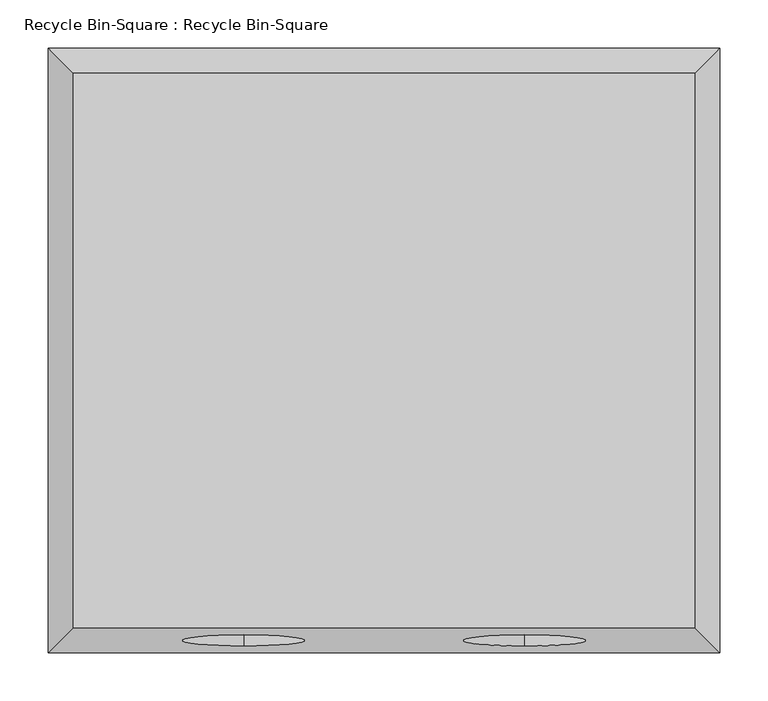
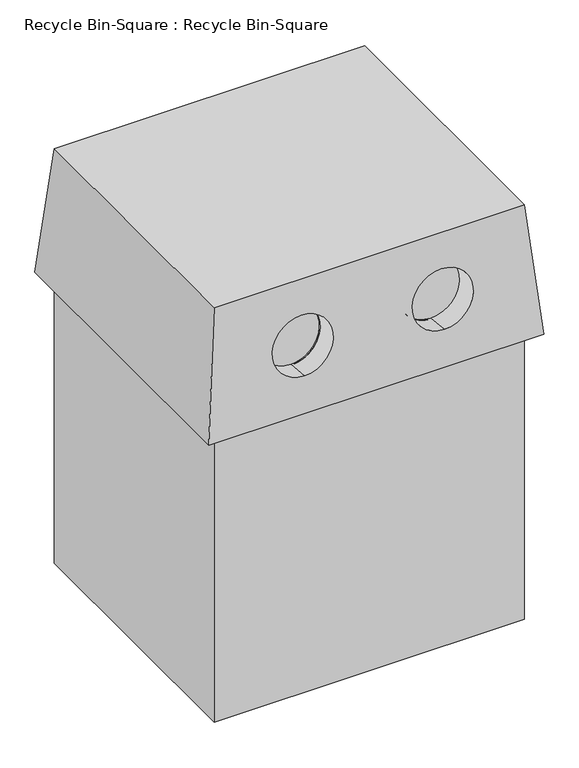
"""IFC4 building model written with IfcOpenShell, lengths in millimetres: proxy geometry, Recycle Bin-Square : Recycle Bin-Square."""

from ifc_helpers import new_model, si_unit, point, frame, frame_2d, origin, origin_with_axes, place, context, project, spatial, polyline, circle_curve, ellipse_curve, trimmed, segment, composite_curve, outline, extrude, source, transform, mapped, element, save
from ifc_brep_helpers import plane_surface, revolved_surface, advanced_brep


def recycle_bin_square_recycle_bin_square_c944da42(model_context):
    return source(origin(), model_context, "Body", "SolidModel", [
        extrude(outline(composite_curve([segment(trimmed(circle_curve(frame_2d((0.0, -63.5)), 63.5), [point((0.0, -127.0))], [point((0.0, 0.0))], False, "CARTESIAN"), True, "CONTINUOUS"), segment(trimmed(circle_curve(frame_2d((0.0, -63.5)), 63.5), [point((0.0, 0.0))], [point((6.35, -0.3182978))], False, "CARTESIAN"), True, "CONTINUOUS"), segment(trimmed(circle_curve(frame_2d((12.7, -63.5)), 63.5), [point((6.35, -0.3182978))], [point((6.35, -126.6817023))], True, "CARTESIAN"), True, "CONTINUOUS"), segment(trimmed(circle_curve(frame_2d((0.0, -63.5)), 63.5), [point((6.35, -126.6817023))], [point((0.0, -127.0))], False, "CARTESIAN"), True, "CONTINUOUS")], self_intersect=False)), frame((-133.35, -251.1401384, 707.756246), z_axis=(0.0, -0.9950371902099875, 0.09950371902101512), x_axis=(-1.0, 0.0, 0.0)), (0.0, 0.0, 1.0), 3.175),
        extrude(outline(composite_curve([segment(trimmed(circle_curve(frame_2d((-266.7, -63.5)), 63.5), [point((-266.7, 0.0))], [point((-266.7, -127.0))], False, "CARTESIAN"), True, "CONTINUOUS"), segment(trimmed(circle_curve(frame_2d((-266.7, -63.5)), 63.5), [point((-266.7, -127.0))], [point((-273.05, -126.6817023))], False, "CARTESIAN"), True, "CONTINUOUS"), segment(trimmed(circle_curve(frame_2d((-279.4, -63.5)), 63.5), [point((-273.05, -126.6817023))], [point((-273.05, -0.3182978))], True, "CARTESIAN"), True, "CONTINUOUS"), segment(trimmed(circle_curve(frame_2d((-266.7, -63.5)), 63.5), [point((-273.05, -0.3182978))], [point((-266.7, 0.0))], False, "CARTESIAN"), True, "CONTINUOUS")], self_intersect=False)), frame((-133.35, -251.1401384, 707.756246), z_axis=(0.0, -0.9950371902099875, 0.09950371902101512), x_axis=(-1.0, 0.0, 0.0)), (0.0, 0.0, 1.0), 3.175),
        extrude(outline(polyline([(323.85, 295.4394238), (323.85, -282.4105762), (-323.85, -282.4105762), (-323.85, 295.4394238), (323.85, 295.4394238)])), origin_with_axes(), (0.0, 0.0, 1.0), 635.0),
        advanced_brep(
        [(323.85, 295.4394238, 914.4), (-323.85, 295.4394238, 914.4), (-323.85, -282.4105762, 914.4), (323.85, -282.4105762, 914.4), (349.25, 320.8394238, 635.0), (349.25, -307.8105762, 635.0), (-349.25, -307.8105762, 635.0), (-349.25, 320.8394238, 635.0), (-146.05, -300.745415, 712.7167737), (-146.05, -289.2469086, 839.2003434), (146.05, -300.745415, 712.7167737), (146.05, -289.2469086, 839.2003434), (-146.05, -238.5031661, 834.1259692), (-146.05, -251.1401384, 707.756246), (146.05, -238.5031661, 834.1259692), (146.05, -251.1401384, 707.756246)],
        [
            (0, 1),
            (1, 2),
            (2, 3),
            (3, 0),
            (4, 5),
            (5, 6),
            (6, 7),
            (7, 4),
            (0, 4),
            (7, 1),
            (6, 2),
            (5, 3),
            (8, 9, ellipse_curve(frame((-146.05, -294.9961618, 775.9585586), z_axis=(0.0, 0.995893206467704, -0.09053574604251848), x_axis=(0.0, 0.09053574604254297, 0.9958932064677015)), 63.5025768, 63.5)),
            (9, 8, ellipse_curve(frame((-146.05, -294.9961618, 775.9585586), z_axis=(0.0, 0.995893206467704, -0.09053574604251848), x_axis=(0.0, 0.09053574604254297, 0.9958932064677015)), 63.5025768, 63.5)),
            (10, 11, ellipse_curve(frame((146.05, -294.9961618, 775.9585586), z_axis=(0.0, 0.995893206467704, -0.09053574604251848), x_axis=(0.0, 0.09053574604254297, 0.9958932064677015)), 63.5025768, 63.5)),
            (11, 10, ellipse_curve(frame((146.05, -294.9961618, 775.9585586), z_axis=(0.0, 0.995893206467704, -0.09053574604251848), x_axis=(0.0, 0.09053574604254297, 0.9958932064677015)), 63.5025768, 63.5)),
            (12, 13, circle_curve(frame((-146.05, -244.8216523, 770.9411076), z_axis=(0.0, -0.9950371902099875, 0.09950371902101512), x_axis=(0.0, -0.09950371902101512, -0.9950371902099875)), 63.5)),
            (13, 12, circle_curve(frame((-146.05, -244.8216523, 770.9411076), z_axis=(0.0, -0.9950371902099875, 0.09950371902101512), x_axis=(0.0, -0.09950371902101512, -0.9950371902099875)), 63.5)),
            (14, 15, circle_curve(frame((146.05, -244.8216523, 770.9411076), z_axis=(0.0, -0.9950371902099875, 0.09950371902101512), x_axis=(0.0, -0.09950371902101512, -0.9950371902099875)), 63.5)),
            (15, 14, circle_curve(frame((146.05, -244.8216523, 770.9411076), z_axis=(0.0, -0.9950371902099875, 0.09950371902101512), x_axis=(0.0, -0.09950371902101512, -0.9950371902099875)), 63.5)),
            (12, 9),
            (8, 13),
            (14, 11),
            (10, 15),
        ],
        [
            plane_surface(frame((0.0, 6.5144238, 914.4), z_axis=(0.0, 0.0, 1.0), x_axis=(-1.0, 0.0, 0.0))),
            plane_surface(frame((0.0, 6.5144238, 635.0), z_axis=(0.0, 0.0, -1.0), x_axis=(-1.0, 0.0, 0.0))),
            plane_surface(frame((0.0, 320.8394238, 635.0), z_axis=(0.0, 0.995893206467704, 0.09053574604251835), x_axis=(-1.0, 0.0, 0.0))),
            plane_surface(frame((-349.25, 6.5144238, 635.0), z_axis=(-0.995893206467703, 0.0, 0.09053574604252924), x_axis=(0.0, -1.0, 0.0))),
            plane_surface(frame((0.0, -307.8105762, 635.0), z_axis=(0.0, -0.995893206467704, 0.09053574604251848), x_axis=(1.0, 0.0, 0.0))),
            plane_surface(frame((349.25, 6.5144238, 635.0), z_axis=(0.9958932064677042, 0.0, 0.09053574604251488), x_axis=(0.0, 1.0, 0.0))),
            plane_surface(frame((-146.05, -251.1401384, 707.756246), z_axis=(0.0, -0.9950371902099875, 0.09950371902101512), x_axis=(-1.0, 0.0, 0.0))),
            revolved_surface(polyline([(-146.05, -301.8838809495378, 712.8306202708369), (-146.05, -251.1401383984275, 707.7562460157251)]), (-146.05, -244.8216523, 770.9411076), (0.0, -0.9950371902099875, 0.09950371902101512)),
            revolved_surface(polyline([(146.05, -301.8838809515181, 712.8306202510341), (146.05, -251.14013840040778, 707.7562459959222)]), (146.05, -295.3695415, 775.9958965), (0.0, -0.9950371902099875, 0.09950371902101512)),
        ],
        [
            (0, [[1, 2, 3, 4]]),
            (1, [[5, 6, 7, 8]]),
            (2, [[-1, 9, -8, 10]]),
            (3, [[-2, -10, -7, 11]]),
            (4, [[-3, -11, -6, 12], [13, 14], [15, 16]]),
            (5, [[-4, -12, -5, -9]]),
            (6, [[17, 18]]),
            (6, [[19, 20]]),
            (7, [[-17, 21, -13, 22]]),
            (7, [[-18, -22, -14, -21]]),
            (8, [[-19, 23, -15, 24]]),
            (8, [[-20, -24, -16, -23]]),
        ],
    ),
    ])


if __name__ == "__main__":
    model = new_model("IFC4")
    model_context = context("Model", 3, world=origin())
    ifc_project = project(units=[si_unit("LENGTHUNIT", "METRE", prefix="MILLI")], contexts=[model_context])
    site = spatial("IfcSite", under=ifc_project)
    building = spatial("IfcBuilding", under=site)
    placement = place(None, origin())
    recycle_bin_square_recycle_bin_square_shape = recycle_bin_square_recycle_bin_square_c944da42(model_context)
    element("IfcBuildingElementProxy", 1, Name="Recycle Bin-Square : Recycle Bin-Square", ObjectType="Recycle Bin-Square : Recycle Bin-Square", at=placement, inside=building, context=model_context, shape_type="MappedRepresentation", body=[
        mapped(recycle_bin_square_recycle_bin_square_shape, transform((0.0, 0.0, 0.0), x_axis=(1.0, 0.0, 0.0), y_axis=(0.0, 1.0, 0.0), z_axis=(0.0, 0.0, 1.0))),
    ])
    save(model, "model.ifc")

# Revit data of these elements
# Type "Recycle Bin-Square : Recycle Bin-Square"
#   Default Elevation = 0
# Element 1 (IfcBuildingElementProxy, "Recycle Bin-Square : Recycle Bin-Square")
#   Materials on its faces: "Plastic - Blue", "Default - Black"
# Materials
#   "Plastic - Blue": class "Plastic", colour RGB 0 0 212, transparency 0
#   "Default - Black": colour RGB 0 0 0, transparency 0
